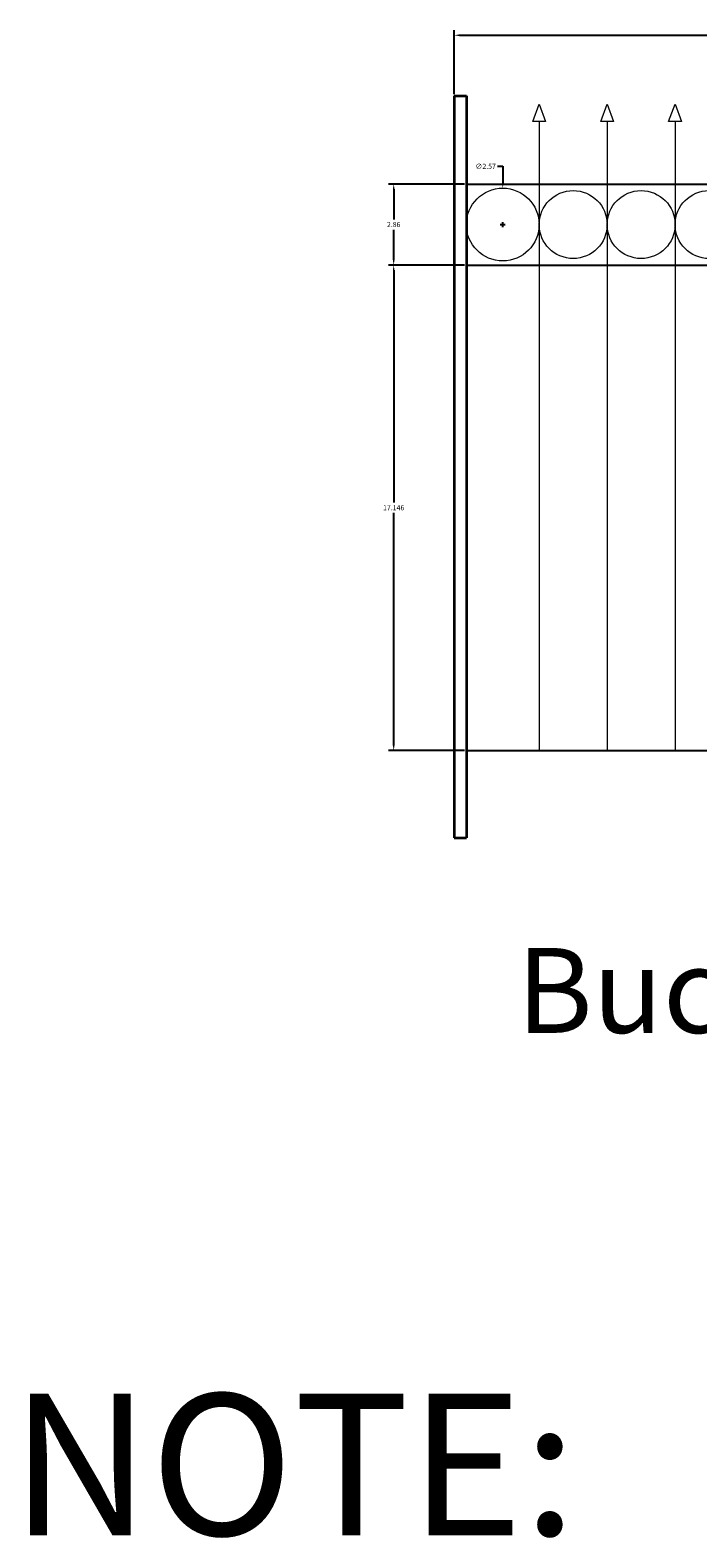
# Model space of a CAD drawing. Units: inches. Extents: x 756 to 915, y 488 to 695.
# Tile 1 of 25: x 756 to 779, y 488 to 541. Entities that reach past the tile are written whole.
import ezdxf

# ---------------------------------------------------------------- set-up
doc = ezdxf.new("R2010")
doc.units = ezdxf.units.IN
doc.header["$MEASUREMENT"] = 0
for name, color, linetype, lineweight in [('L-ANNO-TEXT', 7, 'Continuous', 25), ('L-FENC-PCKT', 7, 'Continuous', 18), ('L-FENC-POST', 7, 'Continuous', 35), ('L-FENC-RAIL', 7, 'Continuous', 25), ('L-FENC-RING', 7, 'Continuous', 18), ('M-DIMS', 2, 'Continuous', 18)]:
    doc.layers.add(name, color=color, linetype=linetype, lineweight=lineweight)
doc.styles.get("Standard").update_dxf_attribs({"font": 'arial.ttf'})
doc.dimstyles.get("Standard").update_dxf_attribs({"dimtxt": 0.18, "dimasz": 0.18, "dimexe": 0.18, "dimexo": 0.0625, "dimgap": 0.09, "dimtad": 0, "dimtih": 1, "dimtoh": 1, "dimdec": 0, "dimzin": 0, "dimdsep": 46, "dimlunit": 3, "dimtxsty": 'Standard', "dimcen": 0.09, "dimadec": 0, "dimazin": 0, "dimtfac": 1, "dimtdec": 0, "dimtofl": 0, "dimtmove": 0, "dimatfit": 3, "dimfxl": 1, "dimtolj": 1, "dimtzin": 0, "dimarcsym": 0})

# ---------------------------------------------------------------- blocks, each defined once
blk = doc.blocks.new('FENCE-POST-LEFT')
for p, q in [((0, 26.207), (0, 0)), ((0, 26.207), (0.426, 26.207)), ((0.426, 26.207), (0.426, 0)), ((0.426, 26.207), (0.426, 0)), ((0, 0), (0.426, 0))]:
    blk.add_line(p, q)
blk = doc.blocks.new('PICKET-SPEAR-FLUSH')
blk.add_line((0.228, 22.215), (0.228, 0))
blk.add_lwpolyline([(0.228, 22.215), (0, 22.215), (0.228, 22.826), (0.455, 22.215)], close=True)
blk = doc.blocks.new('FENCE-PLUS-RING-BAND')
for centre, radius in [((1.286, 1.286), 1.286), ((3.773, 1.286), 1.2), ((6.173, 1.286), 1.2), ((8.572, 1.286), 1.2), ((10.972, 1.286), 1.2), ((13.372, 1.286), 1.2), ((15.772, 1.286), 1.2), ((18.172, 1.286), 1.2), ((20.572, 1.286), 1.2), ((22.972, 1.286), 1.2), ((25.372, 1.286), 1.2), ((27.772, 1.286), 1.2), ((30.172, 1.286), 1.2), ((32.572, 1.286), 1.2), ((34.971, 1.286), 1.2), ((37.388, 1.286), 1.217)]:
    blk.add_circle(centre, radius)
blk = doc.blocks.new('*D72')
at = {"layer": 'Defpoints', "color": 0, "transparency": 16777216}
for p in [(810.347, 540.934), (770.889, 538.794), (810.347, 538.794)]:
    blk.add_point(p, dxfattribs=at)
at = {"layer": 'M-DIMS', "color": 0, "lineweight": -2, "transparency": 16777216}
for p, q in [((770.889, 538.857), (770.889, 541.114)), ((771.069, 540.934), (790.224, 540.934)), ((810.167, 540.934), (791.011, 540.934)), ((810.347, 538.857), (810.347, 541.114))]:
    blk.add_line(p, q, dxfattribs=at)
at = {"layer": 'M-DIMS', "color": 0, "transparency": 16777216}
for points in [[(771.069, 540.964), (771.069, 540.904), (770.889, 540.934)], [(810.167, 540.964), (810.167, 540.904), (810.347, 540.934)]]:
    blk.add_solid(points, dxfattribs=at)
at = {"layer": 'M-DIMS', "color": 0, "transparency": 16777216, "insert": (790.618, 540.934), "char_height": 0.18, "attachment_point": 5}
blk.add_mtext('\\A1;39.46', dxfattribs=at)
blk = doc.blocks.new('*D74')
at = {"layer": 'Defpoints', "color": 0, "transparency": 16777216}
for p in [(768.749, 532.815), (771.315, 532.815), (771.315, 515.669)]:
    blk.add_point(p, dxfattribs=at)
at = {"layer": 'M-DIMS', "color": 0, "lineweight": -2, "transparency": 16777216}
for p, q in [((771.253, 532.815), (768.569, 532.815)), ((768.749, 532.635), (768.749, 524.424)), ((768.749, 515.849), (768.749, 524.06)), ((771.253, 515.669), (768.569, 515.669))]:
    blk.add_line(p, q, dxfattribs=at)
at = {"layer": 'M-DIMS', "color": 0, "transparency": 16777216}
for points in [[(768.719, 532.635), (768.779, 532.635), (768.749, 532.815)], [(768.719, 515.849), (768.779, 515.849), (768.749, 515.669)]]:
    blk.add_solid(points, dxfattribs=at)
at = {"layer": 'M-DIMS', "color": 0, "transparency": 16777216, "insert": (768.749, 524.242), "char_height": 0.18, "attachment_point": 5}
blk.add_mtext('\\A1;17.146', dxfattribs=at)
blk = doc.blocks.new('*D75')
at = {"layer": 'Defpoints', "color": 0, "transparency": 16777216}
for p in [(768.749, 535.679), (771.315, 535.679), (771.315, 532.815)]:
    blk.add_point(p, dxfattribs=at)
at = {"layer": 'M-DIMS', "color": 0, "lineweight": -2, "transparency": 16777216}
for p, q in [((771.253, 535.679), (768.569, 535.679)), ((768.749, 535.499), (768.749, 534.429)), ((768.749, 532.995), (768.749, 534.065)), ((771.253, 532.815), (768.569, 532.815))]:
    blk.add_line(p, q, dxfattribs=at)
at = {"layer": 'M-DIMS', "color": 0, "transparency": 16777216}
for points in [[(768.719, 535.499), (768.779, 535.499), (768.749, 535.679)], [(768.719, 532.995), (768.779, 532.995), (768.749, 532.815)]]:
    blk.add_solid(points, dxfattribs=at)
at = {"layer": 'M-DIMS', "color": 0, "transparency": 16777216, "insert": (768.749, 534.247), "char_height": 0.18, "attachment_point": 5}
blk.add_mtext('\\A1;2.86', dxfattribs=at)
blk = doc.blocks.new('*D84')
at = {"layer": 'Defpoints', "color": 0, "transparency": 16777216}
for p in [(772.6, 535.533), (772.603, 532.961)]:
    blk.add_point(p, dxfattribs=at)
at = {"layer": 'M-DIMS', "color": 0, "lineweight": -2, "transparency": 16777216}
for p, q in [((772.419, 536.305), (772.599, 536.305)), ((772.599, 536.305), (772.6, 535.713)), ((772.511, 534.247), (772.691, 534.247)), ((772.601, 534.157), (772.601, 534.337))]:
    blk.add_line(p, q, dxfattribs=at)
at = {"layer": 'M-DIMS', "color": 0, "transparency": 16777216}
blk.add_solid([(772.63, 535.713), (772.57, 535.713), (772.6, 535.533)], dxfattribs=at)
at = {"layer": 'M-DIMS', "color": 0, "transparency": 16777216, "insert": (771.997, 536.305), "char_height": 0.18, "attachment_point": 5}
blk.add_mtext('\\A1;∅2.57', dxfattribs=at)

msp = doc.modelspace()

# ---------------------------------------------------------------- linework, layer by layer
at = {"layer": 'L-FENC-RAIL'}
for p, q in [((771.3152, 535.6792), (809.92, 535.6792)), ((771.3152, 532.8149), (809.92, 532.8149)), ((771.3152, 515.6691), (809.92, 515.6691))]:
    msp.add_line(p, q, dxfattribs=at)

# ---------------------------------------------------------------- block references
at = {"layer": 'L-FENC-PCKT'}
for p in [(773.66, 515.6687), (776.0599, 515.6687), (778.4598, 515.6687)]:
    msp.add_blockref('PICKET-SPEAR-FLUSH', p, dxfattribs=at)
at = {"layer": 'L-FENC-POST'}
msp.add_blockref('FENCE-POST-LEFT', (770.8889, 512.5874), dxfattribs=at)
at = {"layer": 'L-FENC-RING'}
msp.add_blockref('FENCE-PLUS-RING-BAND', (771.315, 532.961), dxfattribs=at)

# ---------------------------------------------------------------- texts
at = {"layer": 'L-ANNO-TEXT'}
for s, height, p in [('Buckingham Plus', 3, (773.0883, 505.6907)), ('NOTE:', 5, (755.2201, 487.9417))]:
    msp.add_text(s, height=height, dxfattribs=at).set_placement(p)

# ---------------------------------------------------------------- dimensions: what is measured, and where the dimension line sits
at = {"layer": 'M-DIMS'}
dim = msp.add_linear_dim(base=(810.3467, 540.9342), p1=(770.8885, 538.7942), p2=(810.3467, 538.7942), dimstyle='Standard', override={"dimdec": 2, "dimlfac": 1, "dimrnd": 0, "dimzin": 0, "dimdsep": 46, "dimlunit": 2}, dxfattribs=at)
dim.commit()
dim.dimension.update_dxf_attribs({"geometry": '*D72', "text_midpoint": (790.6176, 540.9342)})
dim = msp.add_diameter_dim_2p(p1=(772.6028, 532.9608), p2=(772.6, 535.5333), dimstyle='Standard', override={"dimdec": 2, "dimlfac": 1, "dimrnd": 0, "dimzin": 0, "dimdsep": 46, "dimlunit": 2}, dxfattribs=at)
dim.commit()
dim.dimension.update_dxf_attribs({"geometry": '*D84', "text_midpoint": (771.9974, 536.305), "dimtype": 163})
for base, p1, p2, override, picture, middle in [((768.7485, 535.6792), (771.3152, 532.8149), (771.3152, 535.6792), {"dimdec": 2, "dimlfac": 1, "dimrnd": 0, "dimzin": 0, "dimdsep": 46, "dimlunit": 2}, '*D75', (768.7485, 534.2471)), ((768.7485, 532.8149), (771.3152, 515.6691), (771.3152, 532.8149), {"dimdec": 3, "dimlfac": 1, "dimrnd": 0, "dimzin": 0, "dimdsep": 46, "dimlunit": 2}, '*D74', (768.7485, 524.242))]:
    dim = msp.add_linear_dim(base=base, p1=p1, p2=p2, angle=90, dimstyle='Standard', override=override, dxfattribs=at)
    dim.commit()
    dim.dimension.update_dxf_attribs({"geometry": picture, "text_midpoint": middle})

doc.saveas('drawing.dxf')
